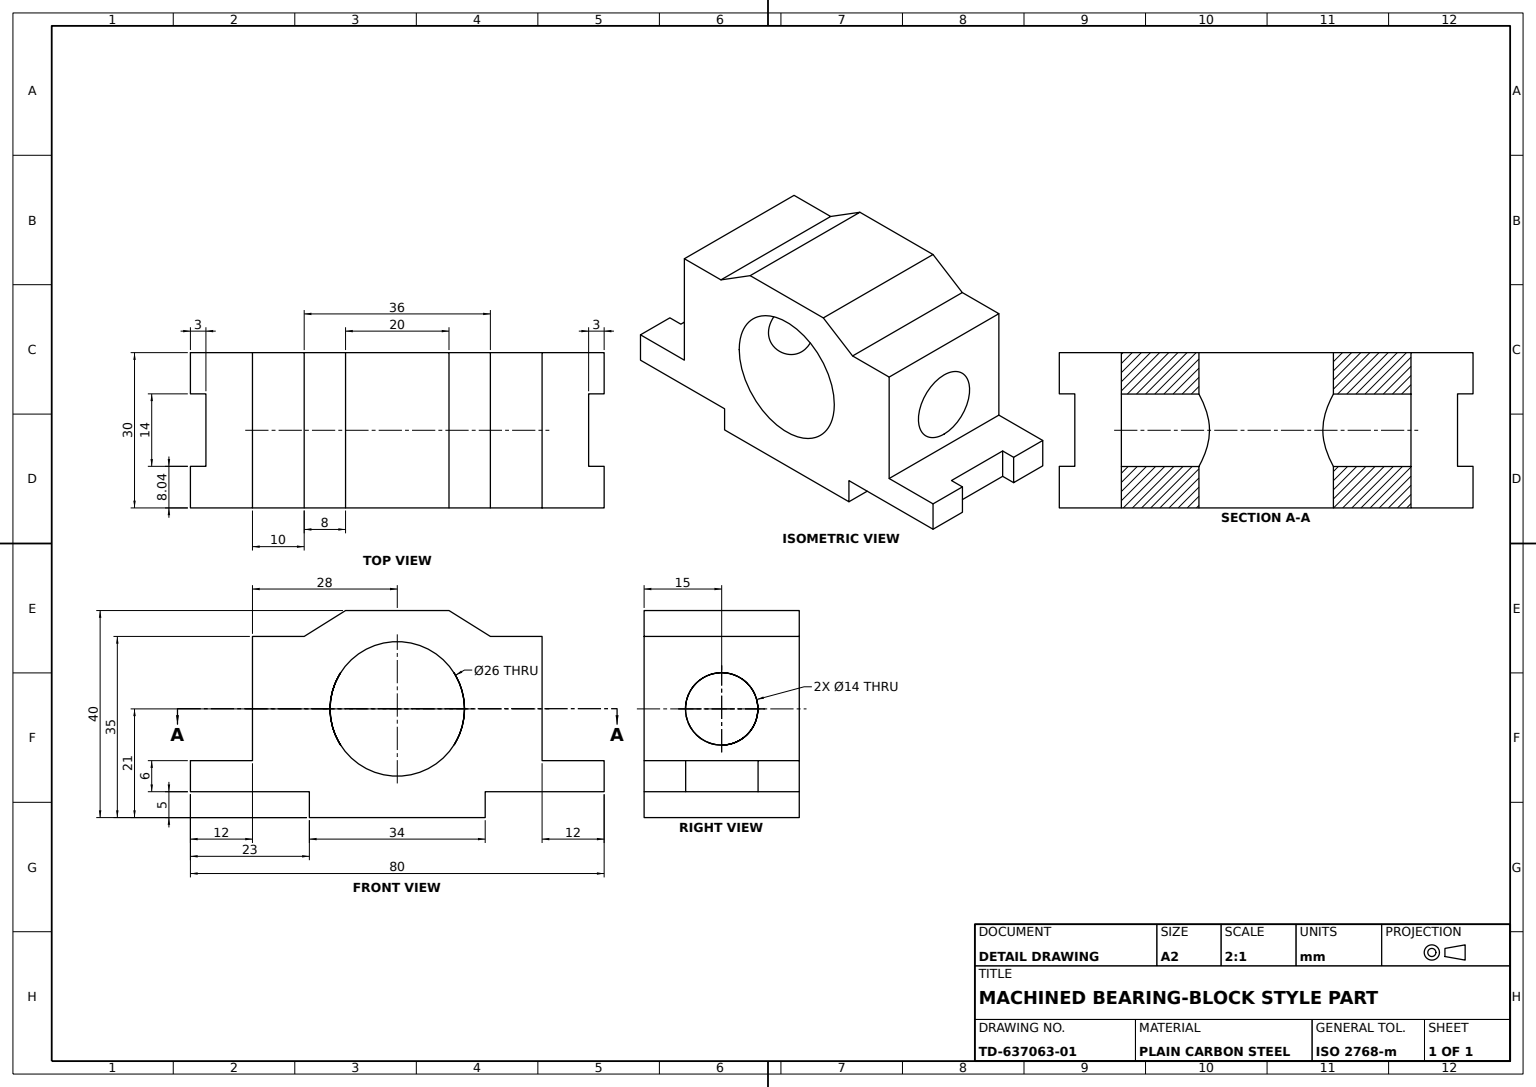
SolidWorks part; units mm, degrees
material "Plain Carbon Steel"
ref_plane "Front Plane" through (0, 0, 0) normal (0, 0, 1) x (1, 0, 0)
ref_plane "Top Plane" through (0, 0, 0) normal (0, 1, 0) x (1, 0, 0)
ref_plane "Right Plane" through (0, 0, 0) normal (1, 0, 0) x (0, 0, -1)
sketch "Block Profile Sketch" plane through (0, 0, 0) normal (0, 0, 1) x (1, 0, 0)
  line L0 (0, 0) -> (23, 0)
  line L1 (23, 0) -> (23, -5)
  line L2 (23, -5) -> (57, -5)
  line L3 (57, -5) -> (57, 0)
  line L4 (57, 0) -> (80, 0)
  line L5 (80, 0) -> (80, 6)
  line L6 (80, 6) -> (68, 6)
  line L7 (68, 6) -> (68, 30)
  line L8 (68, 30) -> (58, 30)
  line L9 (58, 30) -> (50, 35)
  line L10 (50, 35) -> (30, 35)
  line L11 (30, 35) -> (22, 30)
  line L12 (22, 30) -> (12, 30)
  line L13 (12, 30) -> (12, 6)
  line L14 (12, 6) -> (0, 6)
  line L15 (0, 6) -> (0, 0)
  circle A0 centre (40, 16) radius 13
  point P22 (40, -5)
  point P23 (40, 35)
  dimension "D15" = 26
  dimension "D1" = 23
  dimension "D2" = 80
  dimension "D3" = 23
  dimension "D4" = 5
  dimension "D5" = 6
  dimension "D6" = 6
  dimension "D7" = 35
  dimension "D8" = 40
  dimension "D9" = 12
  dimension "D10" = 56
  dimension "D11" = 12
  dimension "D12" = 20
  dimension "D13" = 36
  dimension "D14" = 10
  dimension "D16" = 21
  dimension "D17" = 5
  dimension "D18" = 28
extrude "Block Body" add sketch "Block Profile Sketch" against normal blind 30
sketch "Top Groove Sketch" plane through (0, 6, 0) normal (0, 1, 0) x (1, 0, 0)
  line L0 (0, 8.0371) -> (0, 22.0371)
  line L1 (0, 30) -> (0, 0) construction
  line L2 (0, 22.0371) -> (3, 22.0371)
  line L3 (3, 22.0371) -> (3, 8.0371)
  line L4 (3, 8.0371) -> (0, 8.0371)
  line L5 (12, 30) -> (12, 0) construction
  line L8 (77, 8.0371) -> (80, 8.0371)
  line L9 (77, 22.0371) -> (77, 8.0371)
  line L10 (80, 22.0371) -> (77, 22.0371)
  line L11 (80, 8.0371) -> (80, 22.0371)
  point P5 (0, 15.0371)
  point P17 (80, 15.0371)
  dimension "D1" = 14
  dimension "D2" = 3
  dimension "D3" = 65
  dimension "D4" = 8.0371
extrude "Top Groove Cut" cut sketch "Top Groove Sketch" against normal through all
sketch "Side Cross Hole Sketch" plane through (12, 0, 0) normal (-1, 0, 0) x (0, 0, 1)
  line L0 (-30, 6) -> (0, 6) construction
  circle A0 centre (-15, 16) radius 7
  dimension "D2" = 14
  dimension "D1" = 10
  dimension "D3" = 15
extrude "Side Cross Hole" cut sketch "Side Cross Hole Sketch" against normal through all
